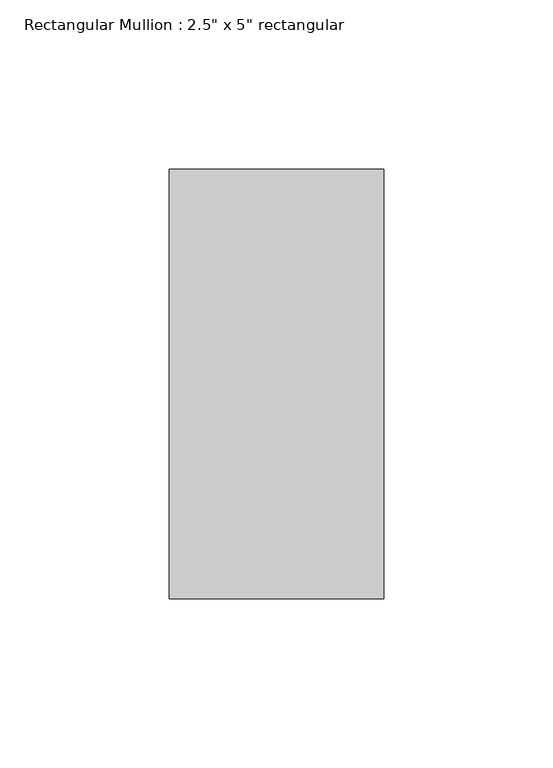
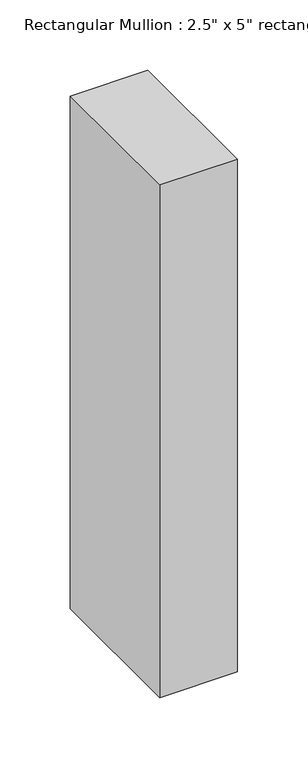
"""IFC4 building model written with IfcOpenShell, lengths in millimetres: member geometry."""

from ifc_helpers import new_model, si_unit, frame, origin, place, context, project, spatial, polyline, outline, extrude, source, transform, mapped, element, save


def member_bc7dbe04(model_context):
    return source(origin(), model_context, "Body", "SweptSolid", [
        extrude(outline(polyline([(0.0, 63.5), (0.0, -63.5), (-63.5, -63.5), (-63.5, 63.5), (0.0, 63.5)])), frame((0.0, 0.0, -444.5), z_axis=(0.0, 0.0, 1.0), x_axis=(1.0, 0.0, 0.0)), (0.0, 0.0, 1.0), 444.5),
    ])


if __name__ == "__main__":
    model = new_model("IFC4")
    model_context = context("Model", 3, world=origin())
    ifc_project = project(units=[si_unit("LENGTHUNIT", "METRE", prefix="MILLI")], contexts=[model_context])
    site = spatial("IfcSite", under=ifc_project)
    building = spatial("IfcBuilding", under=site)
    placement = place(None, origin())
    member_shape = member_bc7dbe04(model_context)
    element("IfcMember", 1, ObjectType="Rectangular Mullion : 2.5\" x 5\" rectangular", at=placement, inside=building, context=model_context, shape_type="MappedRepresentation", body=[
        mapped(member_shape, transform((0.0, 0.0, 0.0), x_axis=(1.0, 0.0, 0.0), y_axis=(0.0, 1.0, 0.0), z_axis=(0.0, 0.0, 1.0))),
    ])
    save(model, "model.ifc")

# Revit data of these elements
# Type "Rectangular Mullion : 2.5\" x 5\" rectangular"
#   built-in parameter 1007304 = 0.416667 (stored number, unit not read)
#   built-in parameter 1007301 = 0.104167 (stored number, unit not read)
#   built-in parameter 1007300 = 0.104167 (stored number, unit not read)
# Element 1 (IfcMember, "Rectangular Mullion : 2.5\" x 5\" rectangular")
#   Materials on its faces: "door colour"
# Materials
#   "door colour": class "Generic", colour RGB 120 120 120, transparency 0, Cost = 0
